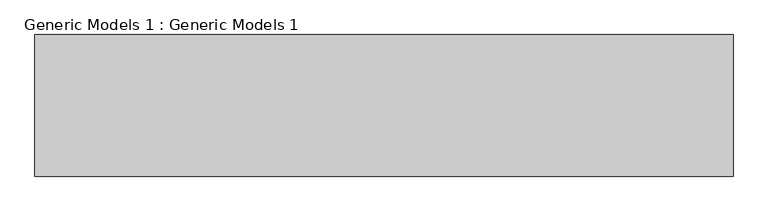
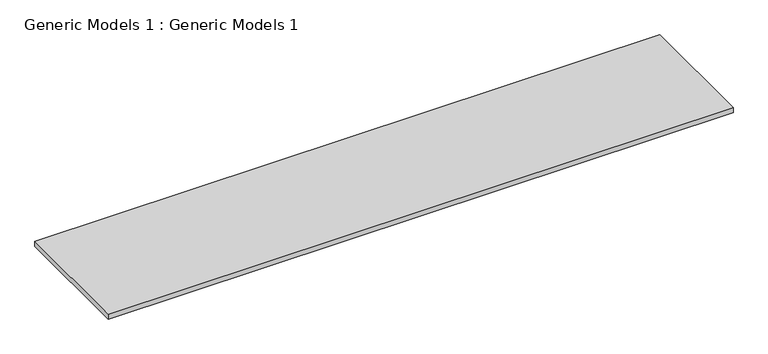
"""IFC4 building model written with IfcOpenShell, lengths in millimetres: proxy geometry, Generic Models 1 : Generic Models 1."""

from ifc_helpers import new_model, si_unit, frame, origin, place, context, project, spatial, polyline, outline, extrude, source, transform, mapped, element, save


def generic_models_1_generic_models_1_3838245b(model_context):
    return source(origin(), model_context, "Body", "SweptSolid", [
        extrude(outline(polyline([(-9655.415666, -15305.8865539), (8632.584334, -15305.8865539), (8632.584334, -19015.7656339), (-9655.415666, -19015.7656339), (-9655.415666, -15305.8865539)])), frame((0.0, 0.0, -152.4), z_axis=(0.0, 0.0, 1.0), x_axis=(1.0, 0.0, 0.0)), (0.0, 0.0, 1.0), 152.4),
    ])


if __name__ == "__main__":
    model = new_model("IFC4")
    model_context = context("Model", 3, world=origin())
    ifc_project = project(units=[si_unit("LENGTHUNIT", "METRE", prefix="MILLI")], contexts=[model_context])
    site = spatial("IfcSite", under=ifc_project)
    building = spatial("IfcBuilding", under=site)
    placement = place(None, origin())
    generic_models_1_generic_models_1_shape = generic_models_1_generic_models_1_3838245b(model_context)
    element("IfcBuildingElementProxy", 1, Name="Generic Models 1 : Generic Models 1", ObjectType="Generic Models 1 : Generic Models 1", at=placement, inside=building, context=model_context, shape_type="MappedRepresentation", body=[
        mapped(generic_models_1_generic_models_1_shape, transform((0.0, 0.0, 0.0), x_axis=(1.0, 0.0, 0.0), y_axis=(0.0, 1.0, 0.0), z_axis=(0.0, 0.0, 1.0))),
    ])
    save(model, "model.ifc")
